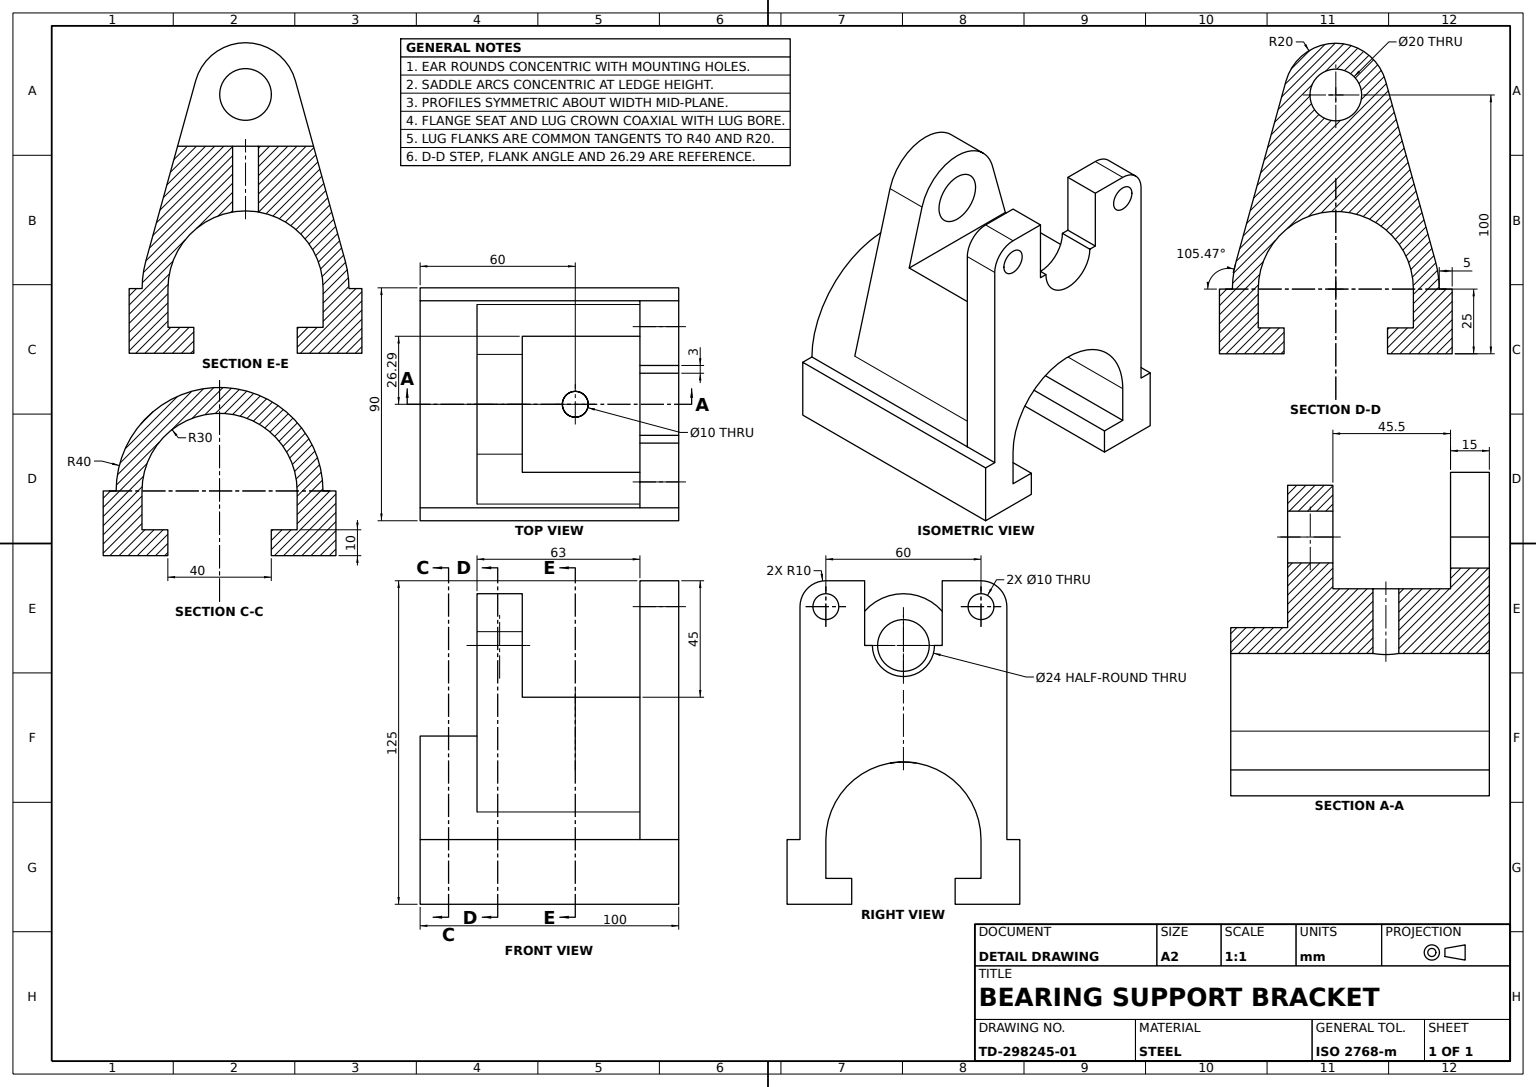
from build123d import *

# Parameters (mm, degrees)
FLANGE_PROFILE_SKETCH_R  = 5
FLANGE_PLATE_15MM_DEPTH  = 15
SADDLE_BODY_100MM_DEPTH  = 100
SUPPORT_BLOCK_SKETCH_R   = 10
SUPPORT_BLOCK_63MM_DEPTH = 63
SLOT_CUT_DEPTH           = 167.282891483
SLOT_CUT_DEPTH_BACK      = 167.282891483
SLOT_CUT_SKETCH_W        = 45.5
SLOT_CUT_SKETCH_H        = 45
CROSS_HOLE_SKETCH_R      = 5
CROSS_HOLE_DEPTH         = 63


with BuildPart() as part:
    # Flange Profile Sketch → Flange Plate 15mm (new body)
    with BuildSketch(Plane.XY):
        with BuildLine():
            ThreePointArc((-12, 100), (0, 88), (12, 100))
            Line((12, 100), (15, 100))
            Line((15, 100), (15, 125))
            Line((15, 125), (30, 125))
            ThreePointArc((30, 125), (37.071067812, 122.071067812), (40, 115))
            Line((40, 115), (40, 25))
            ThreePointArc((40, 25), (0, 65), (-40, 25))
            Line((-40, 25), (-40, 115))
            ThreePointArc((-40, 115), (-37.071067812, 122.071067812), (-30, 125))
            Line((-30, 125), (-15, 125))
            Line((-15, 125), (-15, 100))
            Line((-15, 100), (-12, 100))
        make_face()
        with Locations((-30, 115)):
            Circle(FLANGE_PROFILE_SKETCH_R, mode=Mode.SUBTRACT)
        with Locations((30, 115)):
            Circle(FLANGE_PROFILE_SKETCH_R, mode=Mode.SUBTRACT)
    extrude(amount=FLANGE_PLATE_15MM_DEPTH)

    # Sketch1_4 → Saddle Body 100mm (add)
    with BuildSketch(Plane.XY):
        with BuildLine():
            ThreePointArc((30, 25), (0, 55), (-30, 25))
            Line((-30, 25), (-30, 10))
            Line((-30, 10), (-20, 10))
            Line((-20, 10), (-20, 0))
            Line((-20, 0), (-45, 0))
            Line((-45, 0), (-45, 25))
            Line((-45, 25), (-40, 25))
            ThreePointArc((-40, 25), (0, 65), (40, 25))
            Line((40, 25), (45, 25))
            Line((45, 25), (45, 0))
            Line((45, 0), (20, 0))
            Line((20, 0), (20, 10))
            Line((20, 10), (30, 10))
            Line((30, 10), (30, 25))
        make_face()
    extrude(amount=SADDLE_BODY_100MM_DEPTH)

    # Support Block Sketch → Support Block 63mm (add)
    with BuildSketch(Plane.XY.offset(15)):
        with BuildLine():
            Line((-19.275776393, 105.333333333), (-38.551552786, 35.666666667))
            ThreePointArc((-38.551552786, 35.666666667), (0, 65), (38.551552786, 35.666666667))
            Line((38.551552786, 35.666666667), (19.275776393, 105.333333333))
            ThreePointArc((19.275776393, 105.333333333), (0, 120), (-19.275776393, 105.333333333))
        make_face()
        with Locations((0, 100)):
            Circle(SUPPORT_BLOCK_SKETCH_R, mode=Mode.SUBTRACT)
    extrude(amount=SUPPORT_BLOCK_63MM_DEPTH)

    # Slot Cut Sketch → Slot Cut (cut, two sides: drawn at the far end of the back side and taken through both)
    with BuildSketch(Plane(origin=(0, 0, 0), x_dir=(0, 0, -1), z_dir=(1, 0, 0)).offset(-SLOT_CUT_DEPTH_BACK)):
        with Locations((-37.75, 102.5)):
            Rectangle(SLOT_CUT_SKETCH_W, SLOT_CUT_SKETCH_H)
    extrude(amount=SLOT_CUT_DEPTH + SLOT_CUT_DEPTH_BACK, mode=Mode.SUBTRACT)

    # Cross Hole Sketch → Cross Hole (cut)
    with BuildSketch(Plane(origin=(0, 80, 0), x_dir=(1, 0, 0), z_dir=(0, 1, 0))):
        with Locations(Location((0, -40, 0), (0, 0, 270))):
            Circle(CROSS_HOLE_SKETCH_R)
    extrude(amount=-CROSS_HOLE_DEPTH, mode=Mode.SUBTRACT)


solid = part.part
